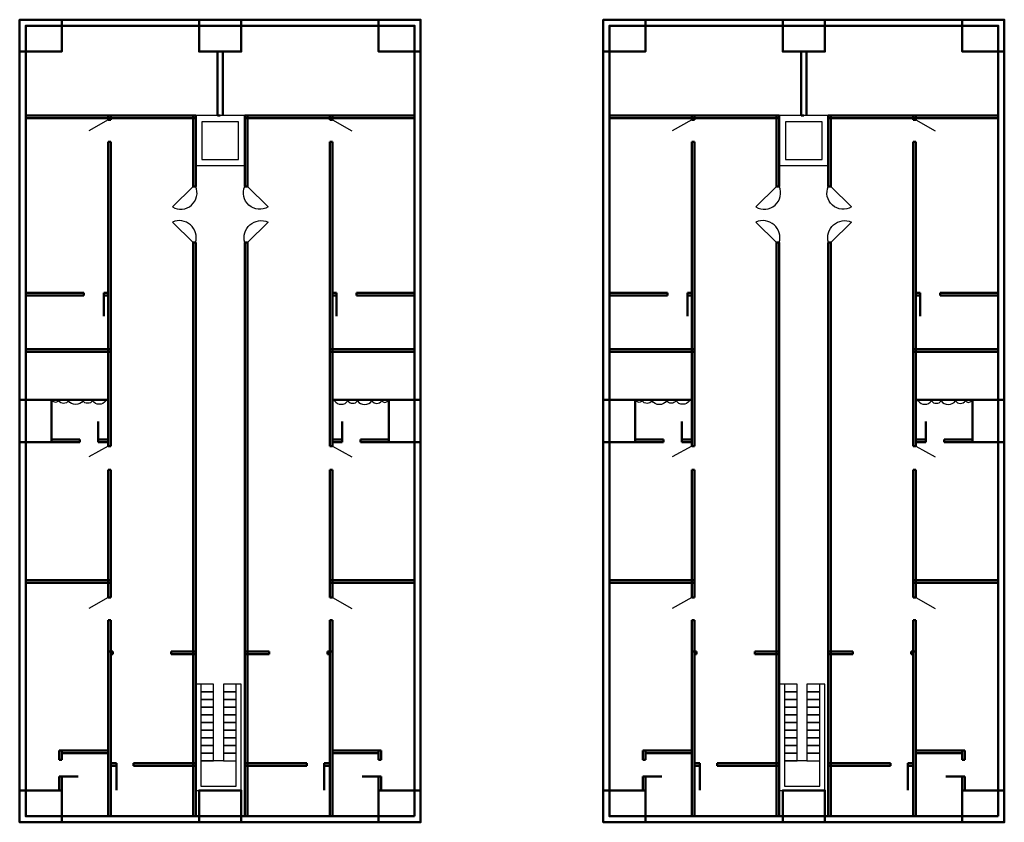
# Model space of a CAD drawing. Units: feet. Extents: x 1080 to 13444, y 870 to 7060.
# Tile 2 of 5: x 4129 to 5603, y 1047 to 2247. Entities that reach past the tile are written whole.
import ezdxf

# ---------------------------------------------------------------- set-up
doc = ezdxf.new("R2010")
doc.units = ezdxf.units.FT
for name, color, linetype, lineweight in [('A-ANNO-NPLT', 8, 'Continuous', 13), ('A-COLS', 1, 'Continuous', 50), ('A-DOOR', 4, 'Continuous', 25), ('A-FLOR-EVTR', 6, 'Continuous', 25), ('A-FLOR-STRS', 2, 'Continuous', 25), ('A-GLAZ', 3, 'Continuous', 25), ('A-WALL', 7, 'Continuous', 50)]:
    doc.layers.add(name, color=color, linetype=linetype, lineweight=lineweight)

# ---------------------------------------------------------------- blocks, each defined once
blk = doc.blocks.new('DOOR-SWING-A')
blk.add_line((30.9, 34), (0, 3.5))
blk.add_arc((12.6, 24.3), 24.3, 238.69, 23.7025)
blk = doc.blocks.new('DOOR-SWING-B')
blk.add_line((0, 30.5), (30.9, 0))
blk.add_arc((10.2, 7), 25.6, 344.0766, 113.531)

msp = doc.modelspace()

# ---------------------------------------------------------------- linework, layer by layer
at = {"layer": 'A-ANNO-NPLT'}
for p in [(4265.6, 1405), (4593.3, 1405), (5138.9, 1405), (5466.5, 1405)]:
    msp.add_point(p, dxfattribs=at)
at = {"layer": 'A-COLS'}
for points in [[(4129.4, 2246.8), (4192.5, 2246.8), (4192.5, 2199.1), (4129.4, 2199.1)], [(4397.9, 2246.8), (4461, 2246.8), (4461, 2199.1), (4397.9, 2199.1)], [(4666.4, 2246.8), (4729.4, 2246.8), (4729.4, 2199.1), (4666.4, 2199.1)], [(5002.7, 2246.8), (5065.7, 2246.8), (5065.7, 2199.1), (5002.7, 2199.1)], [(5271.2, 2246.8), (5334.2, 2246.8), (5334.2, 2199.1), (5271.2, 2199.1)], [(5539.7, 2246.8), (5602.7, 2246.8), (5602.7, 2199.1), (5539.7, 2199.1)], [(4129.4, 1615.2), (4129.4, 1678.3), (4177.1, 1678.3), (4177.1, 1615.2)], [(4729.4, 1678.3), (4729.4, 1615.2), (4681.8, 1615.2), (4681.8, 1678.3)], [(5002.7, 1615.2), (5002.7, 1678.3), (5050.3, 1678.3), (5050.3, 1615.2)], [(5602.7, 1678.3), (5602.7, 1615.2), (5555.1, 1615.2), (5555.1, 1678.3)], [(4192.5, 1094.4), (4129.4, 1094.4), (4129.4, 1046.8), (4192.5, 1046.8)], [(4461, 1046.8), (4397.9, 1046.8), (4397.9, 1094.4), (4461, 1094.4)], [(4666.4, 1094.4), (4729.4, 1094.4), (4729.4, 1046.8), (4666.4, 1046.8)], [(5065.7, 1094.4), (5002.7, 1094.4), (5002.7, 1046.8), (5065.7, 1046.8)], [(5334.2, 1046.8), (5271.2, 1046.8), (5271.2, 1094.4), (5334.2, 1094.4)], [(5539.7, 1094.4), (5602.7, 1094.4), (5602.7, 1046.8), (5539.7, 1046.8)]]:
    msp.add_lwpolyline(points, close=True, dxfattribs=at)
at = {"layer": 'A-DOOR'}
for p, q in [((4261.6, 2096.8), (4232.7, 2080.5)), ((4597.3, 2096.8), (4626.2, 2080.5)), ((5134.9, 2096.8), (5105.9, 2080.5)), ((5470.5, 2096.8), (5499.4, 2080.5)), ((4261.6, 1609.3), (4232.7, 1593)), ((4597.3, 1609.3), (4626.2, 1593)), ((5134.9, 1609.3), (5105.9, 1593)), ((5470.5, 1609.3), (5499.4, 1593)), ((4261.6, 1382.8), (4232.7, 1366.5)), ((4597.3, 1382.8), (4626.2, 1366.5)), ((5134.9, 1382.8), (5105.9, 1366.5)), ((5470.5, 1382.8), (5499.4, 1366.5))]:
    msp.add_line(p, q, dxfattribs=at)
at = {"layer": 'A-FLOR-EVTR'}
for points in [[(4392.8, 2028.8), (4466.1, 2028.8), (4466.1, 2103.4), (4392.8, 2103.4), (4392.8, 2101.1)], [(4401.9, 2037.8), (4457, 2037.8), (4457, 2094.3), (4401.9, 2094.3)], [(5266, 2028.8), (5339.3, 2028.8), (5339.3, 2103.4), (5266, 2103.4), (5266, 2101.1)], [(5275.1, 2037.8), (5330.2, 2037.8), (5330.2, 2094.3), (5275.1, 2094.3)]]:
    msp.add_lwpolyline(points, close=True, dxfattribs=at)
at = {"layer": 'A-FLOR-STRS'}
for points in [[(4400.4, 1253.3), (4392.8, 1253.3), (4392.8, 1094.5), (4460.9, 1094.5), (4460.9, 1253.3), (4453.3, 1253.3)], [(5273.7, 1253.3), (5266, 1253.3), (5266, 1094.5), (5334.2, 1094.5), (5334.2, 1253.3), (5326.5, 1253.3)], [(4434.2, 1138.6), (4400.4, 1138.6), (4400.4, 1100.7), (4453.3, 1100.7), (4453.3, 1138.6)], [(5307.4, 1138.6), (5273.7, 1138.6), (5273.7, 1100.7), (5326.5, 1100.7), (5326.5, 1138.6)]]:
    msp.add_lwpolyline(points, dxfattribs=at)
for points in [[(4400.4, 1253.3), (4400.4, 1241.8), (4419.5, 1241.8), (4419.5, 1253.3)], [(4434.2, 1253.3), (4434.2, 1241.8), (4453.3, 1241.8), (4453.3, 1253.3)], [(5273.7, 1253.3), (5273.7, 1241.8), (5292.8, 1241.8), (5292.8, 1253.3)], [(5307.4, 1253.3), (5307.4, 1241.8), (5326.5, 1241.8), (5326.5, 1253.3)], [(4400.4, 1241.8), (4400.4, 1230.3), (4419.5, 1230.3), (4419.5, 1241.8)], [(4434.2, 1241.8), (4434.2, 1230.3), (4453.3, 1230.3), (4453.3, 1241.8)], [(5273.7, 1241.8), (5273.7, 1230.3), (5292.8, 1230.3), (5292.8, 1241.8)], [(5307.4, 1241.8), (5307.4, 1230.3), (5326.5, 1230.3), (5326.5, 1241.8)], [(4400.4, 1230.3), (4400.4, 1218.9), (4419.5, 1218.9), (4419.5, 1230.3)], [(4434.2, 1230.3), (4434.2, 1218.9), (4453.3, 1218.9), (4453.3, 1230.3)], [(5273.7, 1230.3), (5273.7, 1218.9), (5292.8, 1218.9), (5292.8, 1230.3)], [(5307.4, 1230.3), (5307.4, 1218.9), (5326.5, 1218.9), (5326.5, 1230.3)], [(4400.4, 1218.9), (4400.4, 1207.4), (4419.5, 1207.4), (4419.5, 1218.9)], [(4434.2, 1218.9), (4434.2, 1207.4), (4453.3, 1207.4), (4453.3, 1218.9)], [(5273.7, 1218.9), (5273.7, 1207.4), (5292.8, 1207.4), (5292.8, 1218.9)], [(5307.4, 1218.9), (5307.4, 1207.4), (5326.5, 1207.4), (5326.5, 1218.9)], [(4400.4, 1207.4), (4400.4, 1195.9), (4419.5, 1195.9), (4419.5, 1207.4)], [(4400.4, 1195.9), (4400.4, 1184.5), (4419.5, 1184.5), (4419.5, 1195.9)], [(4434.2, 1207.4), (4434.2, 1195.9), (4453.3, 1195.9), (4453.3, 1207.4)], [(4434.2, 1195.9), (4434.2, 1184.5), (4453.3, 1184.5), (4453.3, 1195.9)], [(5273.7, 1207.4), (5273.7, 1195.9), (5292.8, 1195.9), (5292.8, 1207.4)], [(5273.7, 1195.9), (5273.7, 1184.5), (5292.8, 1184.5), (5292.8, 1195.9)], [(5307.4, 1207.4), (5307.4, 1195.9), (5326.5, 1195.9), (5326.5, 1207.4)], [(5307.4, 1195.9), (5307.4, 1184.5), (5326.5, 1184.5), (5326.5, 1195.9)], [(4400.4, 1184.5), (4400.4, 1173), (4419.5, 1173), (4419.5, 1184.5)], [(4434.2, 1184.5), (4434.2, 1173), (4453.3, 1173), (4453.3, 1184.5)], [(5273.7, 1184.5), (5273.7, 1173), (5292.8, 1173), (5292.8, 1184.5)], [(5307.4, 1184.5), (5307.4, 1173), (5326.5, 1173), (5326.5, 1184.5)], [(4400.4, 1173), (4400.4, 1161.5), (4419.5, 1161.5), (4419.5, 1173)], [(4434.2, 1173), (4434.2, 1161.5), (4453.3, 1161.5), (4453.3, 1173)], [(5273.7, 1173), (5273.7, 1161.5), (5292.8, 1161.5), (5292.8, 1173)], [(5307.4, 1173), (5307.4, 1161.5), (5326.5, 1161.5), (5326.5, 1173)], [(4400.4, 1161.5), (4400.4, 1150.1), (4419.5, 1150.1), (4419.5, 1161.5)], [(4400.4, 1150.1), (4400.4, 1138.6), (4419.5, 1138.6), (4419.5, 1150.1)], [(4434.2, 1161.5), (4434.2, 1150.1), (4453.3, 1150.1), (4453.3, 1161.5)], [(4434.2, 1150.1), (4434.2, 1138.6), (4453.3, 1138.6), (4453.3, 1150.1)], [(5273.7, 1161.5), (5273.7, 1150.1), (5292.8, 1150.1), (5292.8, 1161.5)], [(5273.7, 1150.1), (5273.7, 1138.6), (5292.8, 1138.6), (5292.8, 1150.1)], [(5307.4, 1161.5), (5307.4, 1150.1), (5326.5, 1150.1), (5326.5, 1161.5)], [(5307.4, 1150.1), (5307.4, 1138.6), (5326.5, 1138.6), (5326.5, 1150.1)]]:
    msp.add_lwpolyline(points, close=True, dxfattribs=at)
at = {"layer": 'A-GLAZ'}
for points in [[(4261.3, 1678.3, -0.136738), (4258.3, 1676.9, -0.520567), (4238.3, 1676.9, -0.520567), (4224, 1676.9, -0.520567), (4202.5, 1676.9, -0.520567), (4187.6, 1676.9, -0.520567), (4178.6, 1676.9, -0.053369), (4177.1, 1678.3, -0.053369)], [(4597.6, 1678.3, 0.136738), (4600.6, 1676.9, 0.520567), (4620.6, 1676.9, 0.520567), (4634.9, 1676.9, 0.520567), (4656.4, 1676.9, 0.520567), (4671.3, 1676.9, 0.520567), (4680.2, 1676.9, 0.053369), (4681.8, 1678.3, 0.053369)], [(5134.6, 1678.3, -0.136738), (5131.5, 1676.9, -0.520567), (5111.5, 1676.9, -0.520567), (5097.3, 1676.9, -0.520567), (5075.7, 1676.9, -0.520567), (5060.8, 1676.9, -0.520567), (5051.9, 1676.9, -0.053369), (5050.3, 1678.3, -0.053369)], [(5470.8, 1678.3, 0.136738), (5473.8, 1676.9, 0.520567), (5493.8, 1676.9, 0.520567), (5508.1, 1676.9, 0.520567), (5529.6, 1676.9, 0.520567), (5544.5, 1676.9, 0.520567), (5553.5, 1676.9, 0.053369), (5555.1, 1678.3, 0.053369)]]:
    msp.add_lwpolyline(points, format="xyb", dxfattribs=at)
at = {"layer": 'A-WALL'}
for p, q in [((4425.4, 2103.4), (4425.4, 2199.1)), ((4433.4, 2103.4), (4433.4, 2199.1)), ((5298.7, 2103.4), (5298.7, 2199.1)), ((5306.7, 2103.4), (5306.7, 2199.1)), ((4392.8, 2103.4), (4138.4, 2103.4)), ((4392.8, 2099.4), (4138.4, 2099.4)), ((4261.6, 2103.4), (4261.6, 2096.8)), ((4265.6, 2096.8), (4261.6, 2096.8)), ((4265.6, 2103.4), (4265.6, 2096.8)), ((4388.8, 2103.4), (4388.8, 1997.4)), ((4392.8, 2103.4), (4392.8, 1997.4)), ((4429.4, 2103.4), (4425.4, 2103.4)), ((4466.1, 2103.4), (4720.4, 2103.4)), ((4466.1, 2103.4), (4466.1, 1997.4)), ((4466.1, 2099.4), (4720.4, 2099.4)), ((4470.1, 2103.4), (4470.1, 1997.4)), ((4593.3, 2103.4), (4593.3, 2096.8)), ((4593.3, 2096.8), (4597.3, 2096.8)), ((4597.3, 2103.4), (4597.3, 2096.8)), ((5266, 2103.4), (5011.7, 2103.4)), ((5266, 2099.4), (5011.7, 2099.4)), ((5134.9, 2103.4), (5134.9, 2096.8)), ((5138.9, 2096.8), (5134.9, 2096.8)), ((5138.9, 2103.4), (5138.9, 2096.8)), ((5262, 2103.4), (5262, 1997.4)), ((5266, 2103.4), (5266, 1997.4)), ((5302.7, 2103.4), (5298.7, 2103.4)), ((5339.3, 2103.4), (5593.7, 2103.4)), ((5339.3, 2103.4), (5339.3, 1997.4)), ((5339.3, 2099.4), (5593.7, 2099.4)), ((5343.3, 2103.4), (5343.3, 1997.4)), ((5466.5, 2103.4), (5466.5, 2096.8)), ((5466.5, 2096.8), (5470.5, 2096.8)), ((5470.5, 2103.4), (5470.5, 2096.8)), ((4261.6, 2064.1), (4261.6, 1609.3)), ((4261.6, 2064.1), (4265.6, 2064.1)), ((4265.6, 2064.1), (4265.6, 1609.3)), ((4593.3, 2064.1), (4593.3, 1609.3)), ((4597.3, 2064.1), (4593.3, 2064.1)), ((4597.3, 2064.1), (4597.3, 1609.3)), ((5134.9, 2064.1), (5134.9, 1609.3)), ((5134.9, 2064.1), (5138.9, 2064.1)), ((5138.9, 2064.1), (5138.9, 1609.3)), ((5466.5, 2064.1), (5466.5, 1609.3)), ((5470.5, 2064.1), (5466.5, 2064.1)), ((5470.5, 2064.1), (5470.5, 1609.3)), ((4388.8, 1997.4), (4392.8, 1997.4)), ((4466.1, 1997.4), (4470.1, 1997.4)), ((5262, 1997.4), (5266, 1997.4)), ((5339.3, 1997.4), (5343.3, 1997.4)), ((4388.8, 1913.7), (4388.8, 1302.3)), ((4392.8, 1913.7), (4388.8, 1913.7)), ((4392.8, 1913.7), (4392.8, 1302.3)), ((4466.1, 1913.7), (4466.1, 1302.3)), ((4466.1, 1913.7), (4470.1, 1913.7)), ((4470.1, 1913.7), (4470.1, 1302.3)), ((5262, 1913.7), (5262, 1302.3)), ((5266, 1913.7), (5262, 1913.7)), ((5266, 1913.7), (5266, 1302.3)), ((5339.3, 1913.7), (5339.3, 1302.3)), ((5339.3, 1913.7), (5343.3, 1913.7)), ((5343.3, 1913.7), (5343.3, 1302.3)), ((4138.4, 1754.2), (4138.4, 1838.4)), ((4138.4, 1838.4), (4225.4, 1838.4)), ((4138.4, 1834.4), (4225.4, 1834.4)), ((4225.4, 1838.4), (4225.4, 1834.4)), ((4255.4, 1838.4), (4261.6, 1838.4)), ((4255.4, 1834.4), (4255.4, 1838.4)), ((4255.4, 1834.4), (4261.6, 1834.4)), ((4255.4, 1834.4), (4255.4, 1803.5)), ((4603.5, 1838.4), (4597.3, 1838.4)), ((4603.5, 1834.4), (4597.3, 1834.4)), ((4603.5, 1834.4), (4603.5, 1838.4)), ((4603.5, 1834.4), (4603.5, 1803.5)), ((4720.4, 1838.4), (4633.5, 1838.4)), ((4633.5, 1838.4), (4633.5, 1834.4)), ((4720.4, 1834.4), (4633.5, 1834.4)), ((5011.7, 1754.2), (5011.7, 1838.4)), ((5011.7, 1838.4), (5098.7, 1838.4)), ((5011.7, 1834.4), (5098.7, 1834.4)), ((5098.7, 1838.4), (5098.7, 1834.4)), ((5128.6, 1838.4), (5134.9, 1838.4)), ((5128.6, 1834.4), (5128.6, 1838.4)), ((5128.6, 1834.4), (5134.9, 1834.4)), ((5128.6, 1834.4), (5128.6, 1803.5)), ((5476.7, 1838.4), (5470.5, 1838.4)), ((5476.7, 1834.4), (5470.5, 1834.4)), ((5476.7, 1834.4), (5476.7, 1838.4)), ((5476.7, 1834.4), (5476.7, 1803.5)), ((5593.7, 1838.4), (5506.7, 1838.4)), ((5506.7, 1838.4), (5506.7, 1834.4)), ((5593.7, 1834.4), (5506.7, 1834.4)), ((4265.6, 1754.2), (4138.4, 1754.2)), ((4593.3, 1754.2), (4720.4, 1754.2)), ((5138.9, 1754.2), (5011.7, 1754.2)), ((5466.5, 1754.2), (5593.7, 1754.2)), ((4265.6, 1750.2), (4138.4, 1750.2)), ((4593.3, 1750.2), (4720.4, 1750.2)), ((5138.9, 1750.2), (5011.7, 1750.2)), ((5466.5, 1750.2), (5593.7, 1750.2)), ((4177.1, 1678.3), (4261.6, 1678.3)), ((4681.8, 1678.3), (4597.3, 1678.3)), ((5050.3, 1678.3), (5134.9, 1678.3)), ((5555.1, 1678.3), (5470.5, 1678.3)), ((4246.9, 1619.2), (4246.9, 1646)), ((4612, 1619.2), (4612, 1646)), ((5120.1, 1619.2), (5120.1, 1646)), ((5485.3, 1619.2), (5485.3, 1646)), ((4177.1, 1619.2), (4219.3, 1619.2)), ((4177.1, 1615.2), (4219.3, 1615.2)), ((4219.3, 1619.2), (4219.3, 1615.2)), ((4246.9, 1619.2), (4261.6, 1619.2)), ((4246.9, 1615.2), (4246.9, 1619.2)), ((4246.9, 1615.2), (4261.6, 1615.2)), ((4265.6, 1609.3), (4261.6, 1609.3)), ((4593.3, 1609.3), (4597.3, 1609.3)), ((4612, 1619.2), (4597.3, 1619.2)), ((4612, 1615.2), (4597.3, 1615.2)), ((4612, 1615.2), (4612, 1619.2)), ((4681.8, 1619.2), (4639.6, 1619.2)), ((4639.6, 1619.2), (4639.6, 1615.2)), ((4681.8, 1615.2), (4639.6, 1615.2)), ((5050.3, 1619.2), (5092.6, 1619.2)), ((5050.3, 1615.2), (5092.6, 1615.2)), ((5092.6, 1619.2), (5092.6, 1615.2)), ((5120.1, 1619.2), (5134.9, 1619.2)), ((5120.1, 1615.2), (5120.1, 1619.2)), ((5120.1, 1615.2), (5134.9, 1615.2)), ((5138.9, 1609.3), (5134.9, 1609.3)), ((5466.5, 1609.3), (5470.5, 1609.3)), ((5485.3, 1619.2), (5470.5, 1619.2)), ((5485.3, 1615.2), (5470.5, 1615.2)), ((5485.3, 1615.2), (5485.3, 1619.2)), ((5555.1, 1619.2), (5512.8, 1619.2)), ((5512.8, 1619.2), (5512.8, 1615.2)), ((5555.1, 1615.2), (5512.8, 1615.2)), ((4261.6, 1573.7), (4261.6, 1382.8)), ((4261.6, 1573.7), (4265.6, 1573.7)), ((4265.6, 1573.7), (4265.6, 1382.8)), ((4593.3, 1573.7), (4593.3, 1382.8)), ((4597.3, 1573.7), (4593.3, 1573.7)), ((4597.3, 1573.7), (4597.3, 1382.8)), ((5134.9, 1573.7), (5134.9, 1382.8)), ((5134.9, 1573.7), (5138.9, 1573.7)), ((5138.9, 1573.7), (5138.9, 1382.8)), ((5466.5, 1573.7), (5466.5, 1382.8)), ((5470.5, 1573.7), (5466.5, 1573.7)), ((5470.5, 1573.7), (5470.5, 1382.8)), ((4265.6, 1409), (4138.4, 1409)), ((4265.6, 1405), (4138.4, 1405)), ((4593.3, 1409), (4720.4, 1409)), ((4593.3, 1405), (4720.4, 1405)), ((5138.9, 1409), (5011.7, 1409)), ((5138.9, 1405), (5011.7, 1405)), ((5466.5, 1409), (5593.7, 1409)), ((5466.5, 1405), (5593.7, 1405)), ((4261.6, 1382.8), (4265.6, 1382.8)), ((4597.3, 1382.8), (4593.3, 1382.8)), ((5134.9, 1382.8), (5138.9, 1382.8)), ((5470.5, 1382.8), (5466.5, 1382.8)), ((4261.6, 1348.9), (4261.6, 1302.3)), ((4265.6, 1348.9), (4261.6, 1348.9)), ((4265.6, 1348.9), (4265.6, 1302.3)), ((4593.3, 1348.9), (4593.3, 1302.3)), ((4593.3, 1348.9), (4597.3, 1348.9)), ((4597.3, 1348.9), (4597.3, 1302.3)), ((5134.9, 1348.9), (5134.9, 1302.3)), ((5138.9, 1348.9), (5134.9, 1348.9)), ((5138.9, 1348.9), (5138.9, 1302.3)), ((5466.5, 1348.9), (5466.5, 1302.3)), ((5466.5, 1348.9), (5470.5, 1348.9)), ((5470.5, 1348.9), (5470.5, 1302.3)), ((4261.6, 1055.8), (4261.6, 1302.3)), ((4261.6, 1302.3), (4268.8, 1302.3)), ((4265.6, 1055.8), (4265.6, 1302.3)), ((4265.6, 1298.3), (4268.8, 1298.3)), ((4268.8, 1298.3), (4268.8, 1302.3)), ((4356.3, 1302.3), (4392.8, 1302.3)), ((4356.3, 1302.3), (4356.3, 1298.3)), ((4356.3, 1298.3), (4392.8, 1298.3)), ((4388.8, 1302.3), (4388.8, 1131.4)), ((4392.8, 1302.3), (4392.8, 1131.4)), ((4502.6, 1302.3), (4466.1, 1302.3)), ((4466.1, 1302.3), (4466.1, 1131.4)), ((4502.6, 1298.3), (4466.1, 1298.3)), ((4470.1, 1302.3), (4470.1, 1131.4)), ((4502.6, 1302.3), (4502.6, 1298.3)), ((4597.3, 1302.3), (4590.1, 1302.3)), ((4590.1, 1298.3), (4590.1, 1302.3)), ((4593.3, 1298.3), (4590.1, 1298.3)), ((4593.3, 1055.8), (4593.3, 1302.3)), ((4597.3, 1055.8), (4597.3, 1302.3)), ((5134.9, 1055.8), (5134.9, 1302.3)), ((5134.9, 1302.3), (5142.1, 1302.3)), ((5138.9, 1055.8), (5138.9, 1302.3)), ((5138.9, 1298.3), (5142.1, 1298.3)), ((5142.1, 1298.3), (5142.1, 1302.3)), ((5229.5, 1302.3), (5266, 1302.3)), ((5229.5, 1302.3), (5229.5, 1298.3)), ((5229.5, 1298.3), (5266, 1298.3)), ((5262, 1302.3), (5262, 1131.4)), ((5266, 1302.3), (5266, 1131.4)), ((5375.9, 1302.3), (5339.3, 1302.3)), ((5339.3, 1302.3), (5339.3, 1131.4)), ((5375.9, 1298.3), (5339.3, 1298.3)), ((5343.3, 1302.3), (5343.3, 1131.4)), ((5375.9, 1302.3), (5375.9, 1298.3)), ((5470.5, 1302.3), (5463.3, 1302.3)), ((5463.3, 1298.3), (5463.3, 1302.3)), ((5466.5, 1298.3), (5463.3, 1298.3)), ((5466.5, 1055.8), (5466.5, 1302.3)), ((5470.5, 1055.8), (5470.5, 1302.3)), ((4188.5, 1140.1), (4188.5, 1154.2)), ((4188.5, 1154.2), (4261.6, 1154.2)), ((4192.5, 1140.1), (4192.5, 1154.2)), ((4192.5, 1150.2), (4261.6, 1150.2)), ((4670.4, 1154.2), (4597.3, 1154.2)), ((4666.4, 1150.2), (4597.3, 1150.2)), ((4666.4, 1140.1), (4666.4, 1154.2)), ((4670.4, 1140.1), (4670.4, 1154.2)), ((5061.7, 1140.1), (5061.7, 1154.2)), ((5061.7, 1154.2), (5134.9, 1154.2)), ((5065.7, 1140.1), (5065.7, 1154.2)), ((5065.7, 1150.2), (5134.9, 1150.2)), ((5543.7, 1154.2), (5470.5, 1154.2)), ((5539.7, 1150.2), (5470.5, 1150.2)), ((5539.7, 1140.1), (5539.7, 1154.2)), ((5543.7, 1140.1), (5543.7, 1154.2)), ((4192.5, 1140.1), (4188.5, 1140.1)), ((4274.1, 1135.4), (4265.6, 1135.4)), ((4274.1, 1135.4), (4274.1, 1131.4)), ((4392.8, 1135.4), (4299.6, 1135.4)), ((4299.6, 1131.4), (4299.6, 1135.4)), ((4466.1, 1135.4), (4559.3, 1135.4)), ((4559.3, 1131.4), (4559.3, 1135.4)), ((4584.8, 1135.4), (4593.3, 1135.4)), ((4584.8, 1135.4), (4584.8, 1131.4)), ((4666.4, 1140.1), (4670.4, 1140.1)), ((5065.7, 1140.1), (5061.7, 1140.1)), ((5147.3, 1135.4), (5138.9, 1135.4)), ((5147.3, 1135.4), (5147.3, 1131.4)), ((5266, 1135.4), (5172.8, 1135.4)), ((5172.8, 1131.4), (5172.8, 1135.4)), ((5339.3, 1135.4), (5432.5, 1135.4)), ((5432.5, 1131.4), (5432.5, 1135.4)), ((5458.1, 1135.4), (5466.5, 1135.4)), ((5458.1, 1135.4), (5458.1, 1131.4)), ((5539.7, 1140.1), (5543.7, 1140.1)), ((4274.1, 1131.4), (4265.6, 1131.4)), ((4274.1, 1131.4), (4274.1, 1094.7)), ((4392.8, 1131.4), (4299.6, 1131.4)), ((4388.8, 1131.4), (4388.8, 1055.8)), ((4392.8, 1131.4), (4392.8, 1055.8)), ((4466.1, 1131.4), (4559.3, 1131.4)), ((4466.1, 1131.4), (4466.1, 1055.8)), ((4470.1, 1131.4), (4470.1, 1055.8)), ((4584.8, 1131.4), (4593.3, 1131.4)), ((4584.8, 1131.4), (4584.8, 1094.7)), ((5147.3, 1131.4), (5138.9, 1131.4)), ((5147.3, 1131.4), (5147.3, 1094.7)), ((5266, 1131.4), (5172.8, 1131.4)), ((5262, 1131.4), (5262, 1055.8)), ((5266, 1131.4), (5266, 1055.8)), ((5339.3, 1131.4), (5432.5, 1131.4)), ((5339.3, 1131.4), (5339.3, 1055.8)), ((5343.3, 1131.4), (5343.3, 1055.8)), ((5458.1, 1131.4), (5466.5, 1131.4)), ((5458.1, 1131.4), (5458.1, 1094.7)), ((4188.5, 1094.4), (4188.5, 1115)), ((4188.5, 1115), (4192.5, 1115)), ((4192.5, 1094.4), (4192.5, 1115)), ((4192.5, 1115), (4217, 1115)), ((4666.4, 1115), (4641.9, 1115)), ((4666.4, 1094.4), (4666.4, 1115)), ((4670.4, 1115), (4666.4, 1115)), ((4670.4, 1094.4), (4670.4, 1115)), ((5061.7, 1094.4), (5061.7, 1115)), ((5061.7, 1115), (5065.7, 1115)), ((5065.7, 1094.4), (5065.7, 1115)), ((5065.7, 1115), (5090.3, 1115)), ((5539.7, 1115), (5515.1, 1115)), ((5539.7, 1094.4), (5539.7, 1115)), ((5543.7, 1115), (5539.7, 1115)), ((5543.7, 1094.4), (5543.7, 1115))]:
    msp.add_line(p, q, dxfattribs=at)
for points in [[(4729.4, 1046.8), (4129.4, 1046.8), (4129.4, 2246.8), (4729.4, 2246.8)], [(5602.7, 1046.8), (5002.7, 1046.8), (5002.7, 2246.8), (5602.7, 2246.8)], [(4720.4, 1055.8), (4138.4, 1055.8), (4138.4, 2237.8), (4720.4, 2237.8)], [(5593.7, 1055.8), (5011.7, 1055.8), (5011.7, 2237.8), (5593.7, 2237.8)]]:
    msp.add_lwpolyline(points, close=True, dxfattribs=at)

# ---------------------------------------------------------------- block references
at = {"layer": 'A-DOOR'}
for name, p in [('DOOR-SWING-A', (4357.9, 1963.4)), ('DOOR-SWING-A', (5231.1, 1963.4)), ('DOOR-SWING-B', (4357.9, 1913.7)), ('DOOR-SWING-B', (5231.1, 1913.7))]:
    msp.add_blockref(name, p, dxfattribs=at)
at = {"layer": 'A-DOOR', "extrusion": (0, 0, -1), "zscale": -1, "rotation": 359.9998145993619}
for name, p in [('DOOR-SWING-A', (-4501, 1963.4)), ('DOOR-SWING-A', (-5374.2, 1963.4)), ('DOOR-SWING-B', (-4501, 1913.7)), ('DOOR-SWING-B', (-5374.2, 1913.7))]:
    msp.add_blockref(name, p, dxfattribs=at)

doc.saveas('drawing.dxf')
